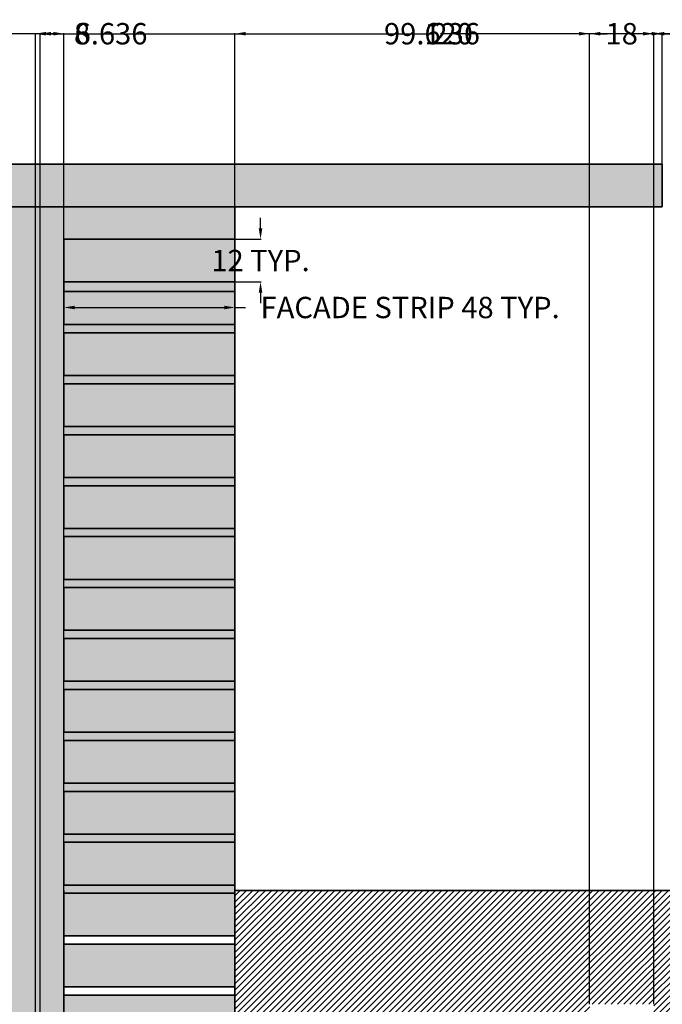
# Model space of a CAD drawing. Units: inches. Extents: x 126 to 726, y 86 to 888.
# Tile 12 of 13: x 426 to 606, y 611 to 888. Entities that reach past the tile are written whole.
import ezdxf

# ---------------------------------------------------------------- set-up
doc = ezdxf.new("R2010")
doc.units = ezdxf.units.IN
doc.header["$MEASUREMENT"] = 0
for name, color, linetype, lineweight in [('A-ANNO-DIMS', 2, 'Continuous', 18), ('A-ELEV', 7, 'Continuous', 35), ('A-ELEV-PATT', 8, 'Continuous', 13)]:
    doc.layers.add(name, color=color, linetype=linetype, lineweight=lineweight)
doc.styles.get("Standard").update_dxf_attribs({"font": 'arial.ttf'})
doc.dimstyles.get("Standard").update_dxf_attribs({"dimtxt": 6, "dimasz": 3, "dimexe": 0.18, "dimexo": 0.0625, "dimgap": 0.09, "dimtad": 0, "dimtih": 1, "dimtoh": 1, "dimdec": 0, "dimzin": 0, "dimdsep": 46, "dimlunit": 3, "dimtxsty": 'Standard', "dimcen": 0.09, "dimadec": 0, "dimazin": 0, "dimtfac": 1, "dimtdec": 0, "dimtofl": 0, "dimtmove": 0, "dimatfit": 3, "dimfxl": 1, "dimtolj": 1, "dimtzin": 0, "dimarcsym": 0})

# ---------------------------------------------------------------- blocks, each defined once
blk = doc.blocks.new('FACADE-STRIP')
for p, q in [((0, 0), (0, 12)), ((0, 12), (48, 12)), ((0, 0), (48, 0))]:
    blk.add_line(p, q)
blk = doc.blocks.new('*D11')
at = {"layer": 'A-ANNO-DIMS', "color": 0, "lineweight": -2, "transparency": 16777216}
for p, q in [((437.97, 813.91), (437.97, 806.6)), ((485.97, 813.91), (485.97, 806.6)), ((440.97, 806.78), (482.97, 806.78)), ((485.97, 806.78), (488.97, 806.78))]:
    blk.add_line(p, q, dxfattribs=at)
at = {"layer": 'A-ANNO-DIMS', "color": 0, "transparency": 16777216}
for points in [[(440.97, 807.28), (440.97, 806.28), (437.97, 806.78)], [(482.97, 807.28), (482.97, 806.28), (485.97, 806.78)]]:
    blk.add_solid(points, dxfattribs=at)
at = {"layer": 'Defpoints', "color": 0, "transparency": 16777216}
for p in [(437.97, 813.98), (485.97, 813.98), (485.97, 806.78)]:
    blk.add_point(p, dxfattribs=at)
at = {"layer": 'A-ANNO-DIMS', "color": 0, "transparency": 16777216, "insert": (535.17, 806.78), "char_height": 6, "attachment_point": 5}
blk.add_mtext('\\A1;FACADE STRIP 48 TYP.', dxfattribs=at)
blk = doc.blocks.new('*D12')
at = {"layer": 'A-ANNO-DIMS', "color": 0, "lineweight": -2, "transparency": 16777216}
for p, q in [((493.17, 828.98), (493.17, 831.98)), ((486.04, 825.98), (493.35, 825.98)), ((486.04, 813.98), (493.35, 813.98)), ((493.17, 810.98), (493.17, 807.98))]:
    blk.add_line(p, q, dxfattribs=at)
at = {"layer": 'A-ANNO-DIMS', "color": 0, "transparency": 16777216}
for points in [[(492.67, 828.98), (493.67, 828.98), (493.17, 825.98)], [(492.67, 810.98), (493.67, 810.98), (493.17, 813.98)]]:
    blk.add_solid(points, dxfattribs=at)
at = {"layer": 'Defpoints', "color": 0, "transparency": 16777216}
for p in [(485.97, 825.98), (493.17, 825.98), (485.97, 813.98)]:
    blk.add_point(p, dxfattribs=at)
at = {"layer": 'A-ANNO-DIMS', "color": 0, "transparency": 16777216, "insert": (493.17, 819.98), "char_height": 6, "attachment_point": 5}
blk.add_mtext('\\A1;12 TYP.', dxfattribs=at)
blk = doc.blocks.new('*D13')
at = {"layer": 'A-ANNO-DIMS', "color": 0, "lineweight": -2, "transparency": 16777216}
for p, q in [((665.97, 642.98), (665.97, 90.21)), ((185.97, 126.98), (185.97, 90.21)), ((188.97, 90.39), (419.15, 90.39)), ((662.97, 90.39), (432.8, 90.39))]:
    blk.add_line(p, q, dxfattribs=at)
at = {"layer": 'A-ANNO-DIMS', "color": 0, "transparency": 16777216}
for points in [[(188.97, 90.89), (188.97, 89.89), (185.97, 90.39)], [(662.97, 90.89), (662.97, 89.89), (665.97, 90.39)]]:
    blk.add_solid(points, dxfattribs=at)
at = {"layer": 'Defpoints', "color": 0, "transparency": 16777216}
for p in [(665.97, 643.04), (185.97, 127.04), (665.97, 90.39)]:
    blk.add_point(p, dxfattribs=at)
at = {"layer": 'A-ANNO-DIMS', "color": 0, "transparency": 16777216, "insert": (425.97, 90.39), "char_height": 6, "attachment_point": 5}
blk.add_mtext('\\A1;480', dxfattribs=at)
blk = doc.blocks.new('*D22')
at = {"layer": 'A-ANNO-DIMS', "color": 0, "lineweight": -2, "transparency": 16777216}
for p, q in [((185.91, 847.04), (149.14, 847.04)), ((149.32, 844.04), (149.32, 708.47)), ((149.32, 566.58), (149.32, 702.16)), ((431.28, 563.58), (149.14, 563.58))]:
    blk.add_line(p, q, dxfattribs=at)
at = {"layer": 'A-ANNO-DIMS', "color": 0, "transparency": 16777216}
for points in [[(148.82, 844.04), (149.82, 844.04), (149.32, 847.04)], [(148.82, 566.58), (149.82, 566.58), (149.32, 563.58)]]:
    blk.add_solid(points, dxfattribs=at)
at = {"layer": 'Defpoints', "color": 0, "transparency": 16777216}
for p in [(149.32, 847.04), (185.97, 847.04), (431.34, 563.58)]:
    blk.add_point(p, dxfattribs=at)
at = {"layer": 'A-ANNO-DIMS', "color": 0, "transparency": 16777216, "insert": (149.32, 705.31), "char_height": 6, "attachment_point": 5}
blk.add_mtext('\\A1;283.46', dxfattribs=at)
blk = doc.blocks.new('*D25')
at = {"layer": 'A-ANNO-DIMS', "color": 0, "lineweight": -2, "transparency": 16777216}
for p, q in [((371.32, 763.42), (371.32, 883.87)), ((374.32, 883.69), (394.42, 883.69)), ((434.97, 883.69), (414.87, 883.69)), ((437.97, 826.04), (437.97, 883.87))]:
    blk.add_line(p, q, dxfattribs=at)
at = {"layer": 'A-ANNO-DIMS', "color": 0, "transparency": 16777216}
for points in [[(374.32, 884.19), (374.32, 883.19), (371.32, 883.69)], [(434.97, 884.19), (434.97, 883.19), (437.97, 883.69)]]:
    blk.add_solid(points, dxfattribs=at)
at = {"layer": 'Defpoints', "color": 0, "transparency": 16777216}
for p in [(437.97, 883.69), (437.97, 825.98), (371.32, 763.35)]:
    blk.add_point(p, dxfattribs=at)
at = {"layer": 'A-ANNO-DIMS', "color": 0, "transparency": 16777216, "insert": (404.65, 883.69), "char_height": 6, "attachment_point": 5}
blk.add_mtext('\\A1;66.66', dxfattribs=at)
blk = doc.blocks.new('*D26')
at = {"layer": 'A-ANNO-DIMS', "color": 0, "lineweight": -2, "transparency": 16777216}
for p, q in [((485.97, 835.1), (485.97, 883.87)), ((488.97, 883.69), (539.55, 883.69)), ((602.97, 883.69), (552.4, 883.69)), ((605.97, 835.1), (605.97, 883.87))]:
    blk.add_line(p, q, dxfattribs=at)
at = {"layer": 'A-ANNO-DIMS', "color": 0, "transparency": 16777216}
for points in [[(488.97, 884.19), (488.97, 883.19), (485.97, 883.69)], [(602.97, 884.19), (602.97, 883.19), (605.97, 883.69)]]:
    blk.add_solid(points, dxfattribs=at)
at = {"layer": 'Defpoints', "color": 0, "transparency": 16777216}
for p in [(605.97, 883.69), (485.97, 835.04), (605.97, 835.04)]:
    blk.add_point(p, dxfattribs=at)
at = {"layer": 'A-ANNO-DIMS', "color": 0, "transparency": 16777216, "insert": (545.97, 883.69), "char_height": 6, "attachment_point": 5}
blk.add_mtext('\\A1;120', dxfattribs=at)
blk = doc.blocks.new('*D41')
at = {"layer": 'A-ANNO-DIMS', "color": 0, "lineweight": -2, "transparency": 16777216}
for p, q in [((429.97, 607.1), (429.97, 883.87)), ((432.97, 883.69), (541.21, 883.69)), ((662.97, 883.69), (554.74, 883.69)), ((665.97, 607.1), (665.97, 883.87))]:
    blk.add_line(p, q, dxfattribs=at)
at = {"layer": 'A-ANNO-DIMS', "color": 0, "transparency": 16777216}
for points in [[(432.97, 884.19), (432.97, 883.19), (429.97, 883.69)], [(662.97, 884.19), (662.97, 883.19), (665.97, 883.69)]]:
    blk.add_solid(points, dxfattribs=at)
at = {"layer": 'Defpoints', "color": 0, "transparency": 16777216}
for p in [(665.97, 883.69), (429.97, 607.04), (665.97, 607.04)]:
    blk.add_point(p, dxfattribs=at)
at = {"layer": 'A-ANNO-DIMS', "color": 0, "transparency": 16777216, "insert": (547.97, 883.69), "char_height": 6, "attachment_point": 5}
blk.add_mtext('\\A1;236', dxfattribs=at)
blk = doc.blocks.new('*D43')
at = {"layer": 'A-ANNO-DIMS', "color": 0, "lineweight": -2, "transparency": 16777216}
for p, q in [((429.97, 595.1), (429.97, 883.87)), ((432.97, 883.69), (434.97, 883.69)), ((437.97, 585.06), (437.97, 883.87)), ((437.97, 883.69), (440.97, 883.69))]:
    blk.add_line(p, q, dxfattribs=at)
at = {"layer": 'A-ANNO-DIMS', "color": 0, "transparency": 16777216}
for points in [[(432.97, 884.19), (432.97, 883.19), (429.97, 883.69)], [(434.97, 884.19), (434.97, 883.19), (437.97, 883.69)]]:
    blk.add_solid(points, dxfattribs=at)
at = {"layer": 'Defpoints', "color": 0, "transparency": 16777216}
for p in [(437.97, 883.69), (429.97, 595.04), (437.97, 585)]:
    blk.add_point(p, dxfattribs=at)
at = {"layer": 'A-ANNO-DIMS', "color": 0, "transparency": 16777216, "insert": (443.04, 883.69), "char_height": 6, "attachment_point": 5}
blk.add_mtext('\\A1;8', dxfattribs=at)
blk = doc.blocks.new('*D44')
at = {"layer": 'A-ANNO-DIMS', "color": 0, "lineweight": -2, "transparency": 16777216}
for p, q in [((431.34, 563.65), (431.34, 883.87)), ((434.34, 883.69), (434.97, 883.69)), ((437.97, 570.75), (437.97, 883.87)), ((437.97, 883.69), (440.97, 883.69))]:
    blk.add_line(p, q, dxfattribs=at)
at = {"layer": 'A-ANNO-DIMS', "color": 0, "transparency": 16777216}
for points in [[(434.34, 884.19), (434.34, 883.19), (431.34, 883.69)], [(434.97, 884.19), (434.97, 883.19), (437.97, 883.69)]]:
    blk.add_solid(points, dxfattribs=at)
at = {"layer": 'Defpoints', "color": 0, "transparency": 16777216}
for p in [(437.97, 883.69), (437.97, 570.69), (431.34, 563.58)]:
    blk.add_point(p, dxfattribs=at)
at = {"layer": 'A-ANNO-DIMS', "color": 0, "transparency": 16777216, "insert": (451.2, 883.69), "char_height": 6, "attachment_point": 5}
blk.add_mtext('\\A1;6.636', dxfattribs=at)
blk = doc.blocks.new('*D50')
at = {"layer": 'A-ANNO-DIMS', "color": 0, "lineweight": -2, "transparency": 16777216}
for p, q in [((485.97, 643.1), (485.97, 883.87)), ((488.97, 883.69), (527.9, 883.69)), ((582.58, 883.69), (543.66, 883.69)), ((585.58, 611.1), (585.58, 883.87))]:
    blk.add_line(p, q, dxfattribs=at)
at = {"layer": 'A-ANNO-DIMS', "color": 0, "transparency": 16777216}
for points in [[(488.97, 884.19), (488.97, 883.19), (485.97, 883.69)], [(582.58, 884.19), (582.58, 883.19), (585.58, 883.69)]]:
    blk.add_solid(points, dxfattribs=at)
at = {"layer": 'Defpoints', "color": 0, "transparency": 16777216}
for p in [(585.58, 883.69), (485.97, 643.04), (585.58, 611.04)]:
    blk.add_point(p, dxfattribs=at)
at = {"layer": 'A-ANNO-DIMS', "color": 0, "transparency": 16777216, "insert": (535.78, 883.69), "char_height": 6, "attachment_point": 5}
blk.add_mtext('\\A1;99.6', dxfattribs=at)
blk = doc.blocks.new('*D51')
at = {"layer": 'A-ANNO-DIMS', "color": 0, "lineweight": -2, "transparency": 16777216}
for p, q in [((585.58, 611.1), (585.58, 883.87)), ((588.58, 883.69), (590.47, 883.69)), ((600.58, 883.69), (598.69, 883.69)), ((603.58, 611.1), (603.58, 883.87))]:
    blk.add_line(p, q, dxfattribs=at)
at = {"layer": 'A-ANNO-DIMS', "color": 0, "transparency": 16777216}
for points in [[(588.58, 884.19), (588.58, 883.19), (585.58, 883.69)], [(600.58, 884.19), (600.58, 883.19), (603.58, 883.69)]]:
    blk.add_solid(points, dxfattribs=at)
at = {"layer": 'Defpoints', "color": 0, "transparency": 16777216}
for p in [(603.58, 883.69), (585.58, 611.04), (603.58, 611.04)]:
    blk.add_point(p, dxfattribs=at)
at = {"layer": 'A-ANNO-DIMS', "color": 0, "transparency": 16777216, "insert": (594.58, 883.69), "char_height": 6, "attachment_point": 5}
blk.add_mtext('\\A1;18', dxfattribs=at)
blk = doc.blocks.new('*D52')
at = {"layer": 'A-ANNO-DIMS', "color": 0, "lineweight": -2, "transparency": 16777216}
for p, q in [((603.58, 611.1), (603.58, 883.87)), ((606.58, 883.69), (608.58, 883.69)), ((611.58, 611.1), (611.58, 883.87)), ((611.58, 883.69), (614.58, 883.69))]:
    blk.add_line(p, q, dxfattribs=at)
at = {"layer": 'A-ANNO-DIMS', "color": 0, "transparency": 16777216}
for points in [[(606.58, 884.19), (606.58, 883.19), (603.58, 883.69)], [(608.58, 884.19), (608.58, 883.19), (611.58, 883.69)]]:
    blk.add_solid(points, dxfattribs=at)
at = {"layer": 'Defpoints', "color": 0, "transparency": 16777216}
for p in [(611.58, 883.69), (603.58, 611.04), (611.58, 611.04)]:
    blk.add_point(p, dxfattribs=at)
at = {"layer": 'A-ANNO-DIMS', "color": 0, "transparency": 16777216, "insert": (616.65, 883.69), "char_height": 6, "attachment_point": 5}
blk.add_mtext('\\A1;8', dxfattribs=at)

msp = doc.modelspace()

# ---------------------------------------------------------------- hatches: boundary and pattern name
at = {"layer": 'A-ELEV-PATT'}
h = msp.add_hatch(color=256, dxfattribs=at)
h.dxf.hatch_style = 1
h.paths.add_polyline_path([(233.9749, 545.5846), (431.3386, 545.5846), (431.3386, 563.5846), (185.9749, 563.5846), (185.9749, 395.5846), (431.3386, 395.5846), (431.3386, 413.5846), (233.9749, 413.5846)])
h.paths.add_polyline_path([(233.9749, 835.0424), (485.9749, 835.0424), (605.9749, 835.0424), (605.9749, 847.0424), (485.9749, 847.0424), (185.9749, 847.0424), (185.9749, 606.5846), (233.9749, 606.5846)])
h.paths.add_polyline_path([(233.9749, 597.5846), (185.9749, 597.5846), (185.9749, 585.5846), (233.9749, 585.5846)])
h.paths.add_polyline_path([(233.9749, 580.5846), (185.9749, 580.5846), (185.9749, 568.5846), (233.9749, 568.5846)])
h = msp.add_hatch(color=256, dxfattribs=at)
h.dxf.hatch_style = 1
h.paths.add_polyline_path([(437.9749, 499.1312), (485.9749, 499.1312), (485.9749, 501.4423), (437.9749, 501.4423), (437.9749, 513.4423), (485.9749, 513.4423), (485.9749, 515.7534), (437.9749, 515.7534), (437.9749, 527.7534), (485.9749, 527.7534), (485.9749, 530.0646), (437.9749, 530.0646), (437.9749, 542.0646), (485.9749, 542.0646), (485.9749, 544.3757), (437.9749, 544.3757), (437.9749, 556.3757), (485.9749, 556.3757), (485.9749, 558.6868), (437.9749, 558.6868), (437.9749, 570.6868), (485.9749, 570.6868), (485.9749, 572.9979), (437.9749, 572.9979), (437.9749, 584.9979), (485.9749, 584.9979), (485.9749, 587.309), (437.9749, 587.309), (437.9749, 595.0424), (429.9749, 595.0424), (429.9749, 607.0424), (437.9749, 607.0424), (437.9749, 615.9312), (437.9749, 630.2423), (437.9749, 642.2423), (485.9749, 642.2423), (485.9749, 644.5534), (437.9749, 644.5534), (437.9749, 656.5534), (485.9749, 656.5534), (485.9749, 658.8645), (437.9749, 658.8645), (437.9749, 670.8645), (485.9749, 670.8645), (485.9749, 673.1757), (437.9749, 673.1757), (437.9749, 685.1757), (485.9749, 685.1757), (485.9749, 687.4868), (437.9749, 687.4868), (437.9749, 699.4868), (485.9749, 699.4868), (485.9749, 701.7979), (437.9749, 701.7979), (437.9749, 713.7979), (485.9749, 713.7979), (485.9749, 716.109), (437.9749, 716.109), (437.9749, 728.109), (485.9749, 728.109), (485.9749, 730.4201), (437.9749, 730.4201), (437.9749, 742.4201), (485.9749, 742.4201), (485.9749, 744.7312), (437.9749, 744.7312), (437.9749, 756.7312), (485.9749, 756.7312), (485.9749, 759.0423), (437.9749, 759.0423), (437.9749, 771.0423), (485.9749, 771.0423), (485.9749, 773.3534), (437.9749, 773.3534), (437.9749, 785.3534), (485.9749, 785.3534), (485.9749, 787.6645), (437.9749, 787.6645), (437.9749, 799.6645), (485.9749, 799.6645), (485.9749, 801.9756), (437.9749, 801.9756), (437.9749, 811.2868), (485.9749, 811.2868), (485.9749, 813.9756), (437.9749, 813.9756), (437.9749, 825.9756), (485.9749, 825.9756), (485.9749, 835.0424), (233.9749, 835.0424), (233.9749, 606.5846), (185.9749, 606.5846), (185.9749, 597.5846), (233.9749, 597.5846), (233.9749, 585.5846), (185.9749, 585.5846), (185.9749, 580.5846), (233.9749, 580.5846), (233.9749, 568.5846), (185.9749, 568.5846), (185.9749, 563.5846), (431.3386, 563.5846), (431.3386, 545.5846), (233.9749, 545.5846), (233.9749, 413.5846), (431.3386, 413.5846), (431.3386, 395.5846), (185.9749, 395.5846), (185.9749, 386.5846), (233.9749, 386.5846), (233.9749, 374.5846), (185.9749, 374.5846), (185.9749, 369.5846), (233.9749, 369.5846), (233.9749, 357.5846), (185.9749, 357.5846), (185.9749, 352.5846), (233.9749, 352.5846), (233.9749, 340.5846), (185.9749, 340.5846), (185.9749, 331.5846), (233.9749, 331.5846), (233.9749, 127.0424), (485.9749, 127.0424), (485.9749, 129.3535), (437.9749, 129.3535), (437.9749, 141.3535), (485.9749, 141.3535), (485.9749, 143.6646), (437.9749, 143.6646), (437.9749, 155.6646), (485.9749, 155.6646), (485.9749, 157.9757), (437.9749, 157.9757), (437.9749, 169.9757), (485.9749, 169.9757), (485.9749, 172.2868), (437.9749, 172.2868), (437.9749, 184.2868), (485.9749, 184.2868), (485.9749, 186.5979), (437.9749, 186.5979), (437.9749, 198.5979), (485.9749, 198.5979), (485.9749, 200.909), (437.9749, 200.909), (437.9749, 212.909), (485.9749, 212.909), (485.9749, 215.2201), (437.9749, 215.2201), (437.9749, 227.2201), (485.9749, 227.2201), (485.9749, 229.5312), (437.9749, 229.5312), (437.9749, 241.5312), (485.9749, 241.5312), (485.9749, 243.8424), (437.9749, 243.8424), (437.9749, 255.8424), (485.9749, 255.8424), (485.9749, 258.1535), (437.9749, 258.1535), (437.9749, 270.1535), (485.9749, 270.1535), (485.9749, 272.4646), (437.9749, 272.4646), (437.9749, 284.4646), (485.9749, 284.4646), (485.9749, 286.7757), (437.9749, 286.7757), (437.9749, 298.7757), (485.9749, 298.7757), (485.9749, 301.0868), (437.9749, 301.0868), (437.9749, 313.0868), (485.9749, 313.0868), (485.9749, 315.3979), (437.9749, 315.3979), (437.9749, 327.3979), (485.9749, 327.3979), (485.9749, 329.709), (437.9749, 329.709), (437.9749, 341.709), (485.9749, 341.709), (485.9749, 344.0201), (437.9749, 344.0201), (437.9749, 355.0424), (429.9749, 355.0424), (429.9749, 367.0424), (437.9749, 367.0424), (437.9749, 372.6423), (437.9749, 386.9535), (437.9749, 401.2646), (437.9749, 413.2646), (485.9749, 413.2646), (485.9749, 415.5757), (437.9749, 415.5757), (437.9749, 427.5757), (485.9749, 427.5757), (485.9749, 429.8868), (437.9749, 429.8868), (437.9749, 441.8868), (485.9749, 441.8868), (485.9749, 444.1979), (437.9749, 444.1979), (437.9749, 456.1979), (485.9749, 456.1979), (485.9749, 458.509), (437.9749, 458.509), (437.9749, 470.509), (485.9749, 470.509), (485.9749, 472.8201), (437.9749, 472.8201), (437.9749, 484.8201), (485.9749, 484.8201), (485.9749, 487.1312), (437.9749, 487.1312)])
h.paths.add_polyline_path([(299.6658, 533.6845), (371.6658, 533.6845), (371.6658, 425.6845), (299.6658, 425.6845)], flags=16)
h.paths.add_polyline_path([(308.6658, 524.6845), (362.6658, 524.6845), (362.6658, 434.6845), (308.6658, 434.6845)], flags=0)
h.paths.add_polyline_path([(317.7956, 603.3211, -0.4129833), (306.8418, 614.321, -0.94403766), (328.769, 615.5845, -0.04423165), (330.7031, 615.4048, -0.89973713), (352.5798, 615.6161, -0.4129833), (363.5336, 604.6162, -0.94403766), (341.6064, 603.3528, -0.04423165), (339.6723, 603.5324, -0.89973713)], flags=16)
h.paths.add_polyline_path([(319.7228, 604.5846, -0.02633223), (319.7726, 605.5306, -0.47905713), (308.8418, 614.321, -1), (326.8418, 614.321, -0.02633223), (326.7919, 613.375, -0.17413188), (332.826, 612.5948, -0.04918553), (332.6526, 614.3527, -1), (350.6526, 614.3527, -0.02633223), (350.6028, 613.4067, -0.47905713), (361.5336, 604.6162, -1), (343.5336, 604.6162, -0.02633223), (343.5834, 605.5622, -0.17413188), (337.5494, 606.3424, -0.04918553), (337.7228, 604.5846, -1)], flags=0)
h.paths.add_polyline_path([(328.769, 355.6561, -0.04423165), (330.7031, 355.4765, -0.89973713), (352.5798, 355.6878, -0.4129833), (363.5336, 344.6879, -0.94403766), (341.6064, 343.4244, -0.04423165), (339.6723, 343.604, -0.89973713), (317.7956, 343.3927, -0.4129833), (306.8418, 354.3926, -0.94403766)], flags=16)
h.paths.add_polyline_path([(326.8418, 354.3926, -0.02633223), (326.7919, 353.4466, -0.17413188), (332.826, 352.6664, -0.04918553), (332.6526, 354.4243, -1), (350.6526, 354.4243, -0.02633223), (350.6028, 353.4783, -0.47905713), (361.5336, 344.6879, -1), (343.5336, 344.6879, -0.02633223), (343.5834, 345.6339, -0.17413188), (337.5494, 346.4141, -0.04918553), (337.7228, 344.6562, -1), (319.7228, 344.6562, -0.02633223), (319.7726, 345.6022, -0.47905713), (308.8418, 354.3926, -1)], flags=0)
h.paths.add_polyline_path([(299.3189, 655.3527), (299.3189, 763.3527), (371.3189, 763.3527), (371.3189, 655.3527)], flags=16)
h.paths.add_polyline_path([(308.3189, 664.3527), (308.3189, 754.3527), (362.3189, 754.3527), (362.3189, 664.3527)], flags=0)
h.paths.add_polyline_path([(299.6658, 303.5875), (371.6658, 303.5875), (371.6658, 195.5875), (299.6658, 195.5875)], flags=16)
h.paths.add_polyline_path([(308.6658, 294.5875), (362.6658, 294.5875), (362.6658, 204.5875), (308.6658, 204.5875)], flags=0)
h.paths.add_polyline_path([(326.3038, 177.3867), (346.055, 177.3867, -0.41421356), (349.055, 174.3867), (349.055, 171.2378), (363.489, 171.2378, -0.41421356), (366.489, 168.2378), (366.489, 159.7133, -0.41421356), (363.489, 156.7133), (343.7379, 156.7133, -0.41421356), (340.7379, 159.7133), (340.7379, 162.8622), (330.5504, 162.8622), (330.5504, 159.7133, -0.41421356), (327.5504, 156.7133), (307.7992, 156.7133, -0.41421356), (304.7992, 159.7133), (304.7992, 168.2378, -0.41421356), (307.7992, 171.2378), (323.3038, 171.2378), (323.3038, 174.3867, -0.41421356)], flags=16)
h.paths.add_polyline_path([(326.3038, 175.3867), (346.055, 175.3867, -0.41421356), (347.055, 174.3867), (347.055, 169.2378), (363.489, 169.2378, -0.41421356), (364.489, 168.2378), (364.489, 159.7133, -0.41421356), (363.489, 158.7133), (343.7379, 158.7133, -0.41421356), (342.7379, 159.7133), (342.7379, 164.8622), (328.5504, 164.8622), (328.5504, 159.7133, -0.41421356), (327.5504, 158.7133), (307.7992, 158.7133, -0.41421356), (306.7992, 159.7133), (306.7992, 168.2378, -0.41421356), (307.7992, 169.2378), (325.3038, 169.2378), (325.3038, 174.3867, -0.41421356)], flags=0)
h = msp.add_hatch(dxfattribs=at)
h.set_pattern_fill('GRAVEL', color=256, scale=40)
h.paths.add_polyline_path([(437.9749, 642.2423), (485.9749, 642.2423), (485.9749, 644.5534), (437.9749, 644.5534), (437.9749, 656.5534), (485.9749, 656.5534), (485.9749, 658.8645), (437.9749, 658.8645), (437.9749, 670.8645), (485.9749, 670.8645), (485.9749, 673.1757), (437.9749, 673.1757), (437.9749, 685.1757), (485.9749, 685.1757), (485.9749, 687.4868), (437.9749, 687.4868), (437.9749, 699.4868), (485.9749, 699.4868), (485.9749, 701.7979), (437.9749, 701.7979), (437.9749, 713.7979), (485.9749, 713.7979), (485.9749, 716.109), (437.9749, 716.109), (437.9749, 728.109), (485.9749, 728.109), (485.9749, 730.4201), (437.9749, 730.4201), (437.9749, 742.4201), (485.9749, 742.4201), (485.9749, 744.7312), (437.9749, 744.7312), (437.9749, 756.7312), (485.9749, 756.7312), (485.9749, 759.0423), (437.9749, 759.0423), (437.9749, 771.0423), (485.9749, 771.0423), (485.9749, 773.3534), (437.9749, 773.3534), (437.9749, 785.3534), (485.9749, 785.3534), (485.9749, 787.6645), (437.9749, 787.6645), (437.9749, 799.6645), (485.9749, 799.6645), (485.9749, 801.9756), (437.9749, 801.9756), (437.9749, 811.2868), (485.9749, 811.2868), (485.9749, 813.9756), (437.9749, 813.9756), (437.9749, 825.9756), (485.9749, 825.9756), (485.9749, 835.0424), (233.9749, 835.0424), (233.9749, 606.5846), (185.9749, 606.5846), (185.9749, 597.5846), (233.9749, 597.5846), (233.9749, 585.5846), (185.9749, 585.5846), (185.9749, 580.5846), (233.9749, 580.5846), (233.9749, 568.5846), (185.9749, 568.5846), (185.9749, 563.5846), (431.3386, 563.5846), (431.3386, 545.5846), (233.9749, 545.5846), (233.9749, 413.5846), (431.3386, 413.5846), (431.3386, 395.5846), (185.9749, 395.5846), (185.9749, 386.5846), (233.9749, 386.5846), (233.9749, 374.5846), (185.9749, 374.5846), (185.9749, 369.5846), (233.9749, 369.5846), (233.9749, 357.5846), (185.9749, 357.5846), (185.9749, 352.5846), (233.9749, 352.5846), (233.9749, 340.5846), (185.9749, 340.5846), (185.9749, 331.5846), (233.9749, 331.5846), (233.9749, 127.0424), (485.9749, 127.0424), (485.9749, 129.3535), (437.9749, 129.3535), (437.9749, 141.3535), (485.9749, 141.3535), (485.9749, 143.6646), (437.9749, 143.6646), (437.9749, 155.6646), (485.9749, 155.6646), (485.9749, 157.9757), (437.9749, 157.9757), (437.9749, 169.9757), (485.9749, 169.9757), (485.9749, 172.2868), (437.9749, 172.2868), (437.9749, 184.2868), (485.9749, 184.2868), (485.9749, 186.5979), (437.9749, 186.5979), (437.9749, 198.5979), (485.9749, 198.5979), (485.9749, 200.909), (437.9749, 200.909), (437.9749, 212.909), (485.9749, 212.909), (485.9749, 215.2201), (437.9749, 215.2201), (437.9749, 227.2201), (485.9749, 227.2201), (485.9749, 229.5312), (437.9749, 229.5312), (437.9749, 241.5312), (485.9749, 241.5312), (485.9749, 243.8424), (437.9749, 243.8424), (437.9749, 255.8424), (485.9749, 255.8424), (485.9749, 258.1535), (437.9749, 258.1535), (437.9749, 270.1535), (485.9749, 270.1535), (485.9749, 272.4646), (437.9749, 272.4646), (437.9749, 284.4646), (485.9749, 284.4646), (485.9749, 286.7757), (437.9749, 286.7757), (437.9749, 298.7757), (485.9749, 298.7757), (485.9749, 301.0868), (437.9749, 301.0868), (437.9749, 313.0868), (485.9749, 313.0868), (485.9749, 315.3979), (437.9749, 315.3979), (437.9749, 327.3979), (485.9749, 327.3979), (485.9749, 329.709), (437.9749, 329.709), (437.9749, 341.709), (485.9749, 341.709), (485.9749, 344.0201), (437.9749, 344.0201), (437.9749, 355.0424), (429.9749, 355.0424), (429.9749, 367.0424), (437.9749, 367.0424), (437.9749, 372.6423), (437.9749, 386.9535), (437.9749, 401.2646), (437.9749, 413.2646), (485.9749, 413.2646), (485.9749, 415.5757), (437.9749, 415.5757), (437.9749, 427.5757), (485.9749, 427.5757), (485.9749, 429.8868), (437.9749, 429.8868), (437.9749, 441.8868), (485.9749, 441.8868), (485.9749, 444.1979), (437.9749, 444.1979), (437.9749, 456.1979), (485.9749, 456.1979), (485.9749, 458.509), (437.9749, 458.509), (437.9749, 470.509), (485.9749, 470.509), (485.9749, 472.8201), (437.9749, 472.8201), (437.9749, 484.8201), (485.9749, 484.8201), (485.9749, 487.1312), (437.9749, 487.1312), (437.9749, 499.1312), (485.9749, 499.1312), (485.9749, 501.4423), (437.9749, 501.4423), (437.9749, 513.4423), (485.9749, 513.4423), (485.9749, 515.7534), (437.9749, 515.7534), (437.9749, 527.7534), (485.9749, 527.7534), (485.9749, 530.0646), (437.9749, 530.0646), (437.9749, 542.0646), (485.9749, 542.0646), (485.9749, 544.3757), (437.9749, 544.3757), (437.9749, 556.3757), (485.9749, 556.3757), (485.9749, 558.6868), (437.9749, 558.6868), (437.9749, 570.6868), (485.9749, 570.6868), (485.9749, 572.9979), (437.9749, 572.9979), (437.9749, 584.9979), (485.9749, 584.9979), (485.9749, 587.309), (437.9749, 587.309), (437.9749, 595.0424), (429.9749, 595.0424), (429.9749, 607.0424), (437.9749, 607.0424), (437.9749, 615.9312), (437.9749, 630.2423)])
h.paths.add_polyline_path([(371.3189, 655.3527), (299.3189, 655.3527), (299.3189, 763.3527), (371.3189, 763.3527)], flags=16)
h.paths.add_polyline_path([(363.5336, 604.6162, -0.94403766), (341.6064, 603.3528, -0.04423165), (339.6723, 603.5324, -0.89973713), (317.7956, 603.3211, -0.4129833), (306.8418, 614.321, -0.94403766), (328.769, 615.5845, -0.04423165), (330.7031, 615.4048, -0.89973713), (352.5798, 615.6161, -0.4129833)], flags=16)
h.paths.add_polyline_path([(361.5336, 604.6162, -1), (343.5336, 604.6162, -0.02633223), (343.5834, 605.5622, -0.17413188), (337.5494, 606.3424, -0.04918553), (337.7228, 604.5846, -1), (319.7228, 604.5846, -0.02633223), (319.7726, 605.5306, -0.47905713), (308.8418, 614.321, -1), (326.8418, 614.321, -0.02633223), (326.7919, 613.375, -0.17413188), (332.826, 612.5948, -0.04918553), (332.6526, 614.3527, -1), (350.6526, 614.3527, -0.02633223), (350.6028, 613.4067, -0.47905713)], flags=0)
h.paths.add_polyline_path([(362.3189, 664.3527), (308.3189, 664.3527), (308.3189, 754.3527), (362.3189, 754.3527)], flags=0)
h.paths.add_polyline_path([(371.6658, 533.6845), (371.6658, 425.6845), (299.6658, 425.6845), (299.6658, 533.6845)], flags=16)
h.paths.add_polyline_path([(362.6658, 524.6845), (362.6658, 434.6845), (308.6658, 434.6845), (308.6658, 524.6845)], flags=0)
h.paths.add_polyline_path([(352.5798, 355.6878, -0.4129833), (363.5336, 344.6879, -0.94403766), (341.6064, 343.4244, -0.04423165), (339.6723, 343.604, -0.89973713), (317.7956, 343.3927, -0.4129833), (306.8418, 354.3926, -0.94403766), (328.769, 355.6561, -0.04423165), (330.7031, 355.4765, -0.89973713)], flags=16)
h.paths.add_polyline_path([(350.6526, 354.4243, -0.02633223), (350.6028, 353.4783, -0.47905713), (361.5336, 344.6879, -1), (343.5336, 344.6879, -0.02633223), (343.5834, 345.6339, -0.17413188), (337.5494, 346.4141, -0.04918553), (337.7228, 344.6562, -1), (319.7228, 344.6562, -0.02633223), (319.7726, 345.6022, -0.47905713), (308.8418, 354.3926, -1), (326.8418, 354.3926, -0.02633223), (326.7919, 353.4466, -0.17413188), (332.826, 352.6664, -0.04918553), (332.6526, 354.4243, -1)], flags=0)
h.paths.add_polyline_path([(371.6658, 303.5875), (371.6658, 195.5875), (299.6658, 195.5875), (299.6658, 303.5875)], flags=16)
h.paths.add_polyline_path([(362.6658, 294.5875), (362.6658, 204.5875), (308.6658, 204.5875), (308.6658, 294.5875)], flags=0)
h.paths.add_polyline_path([(346.055, 177.3867, -0.41421356), (349.055, 174.3867), (349.055, 171.2378), (363.489, 171.2378, -0.41421356), (366.489, 168.2378), (366.489, 159.7133, -0.41421356), (363.489, 156.7133), (343.7379, 156.7133, -0.41421356), (340.7379, 159.7133), (340.7379, 162.8622), (330.5504, 162.8622), (330.5504, 159.7133, -0.41421356), (327.5504, 156.7133), (307.7992, 156.7133, -0.41421356), (304.7992, 159.7133), (304.7992, 168.2378, -0.41421356), (307.7992, 171.2378), (323.3038, 171.2378), (323.3038, 174.3867, -0.41421356), (326.3038, 177.3867)], flags=16)
h.paths.add_polyline_path([(346.055, 175.3867, -0.41421356), (347.055, 174.3867), (347.055, 169.2378), (363.489, 169.2378, -0.41421356), (364.489, 168.2378), (364.489, 159.7133, -0.41421356), (363.489, 158.7133), (343.7379, 158.7133, -0.41421356), (342.7379, 159.7133), (342.7379, 164.8622), (328.5504, 164.8622), (328.5504, 159.7133, -0.41421356), (327.5504, 158.7133), (307.7992, 158.7133, -0.41421356), (306.7992, 159.7133), (306.7992, 168.2378, -0.41421356), (307.7992, 169.2378), (325.3038, 169.2378), (325.3038, 174.3867, -0.41421356), (326.3038, 175.3867)], flags=0)
h = msp.add_hatch(color=256, dxfattribs=at)
h.dxf.hatch_style = 1
h.paths.add_polyline_path([(485.9749, 427.5757), (437.9749, 427.5757), (437.9749, 415.5757), (485.9749, 415.5757)])
h.paths.add_polyline_path([(485.9749, 441.8868), (437.9749, 441.8868), (437.9749, 429.8868), (485.9749, 429.8868)])
h.paths.add_polyline_path([(485.9749, 456.1979), (437.9749, 456.1979), (437.9749, 444.1979), (485.9749, 444.1979)])
h.paths.add_polyline_path([(485.9749, 470.509), (437.9749, 470.509), (437.9749, 458.509), (485.9749, 458.509)])
h.paths.add_polyline_path([(485.9749, 484.8201), (437.9749, 484.8201), (437.9749, 472.8201), (485.9749, 472.8201)])
h.paths.add_polyline_path([(485.9749, 499.1312), (437.9749, 499.1312), (437.9749, 487.1312), (485.9749, 487.1312)])
h.paths.add_polyline_path([(485.9749, 513.4423), (437.9749, 513.4423), (437.9749, 501.4423), (485.9749, 501.4423)])
h.paths.add_polyline_path([(485.9749, 527.7534), (437.9749, 527.7534), (437.9749, 515.7534), (485.9749, 515.7534)])
h.paths.add_polyline_path([(485.9749, 542.0646), (437.9749, 542.0646), (437.9749, 530.0646), (485.9749, 530.0646)])
h.paths.add_polyline_path([(485.9749, 556.3757), (437.9749, 556.3757), (437.9749, 544.3757), (485.9749, 544.3757)])
h.paths.add_polyline_path([(485.9749, 570.6868), (437.9749, 570.6868), (437.9749, 558.6868), (485.9749, 558.6868)])
h.paths.add_polyline_path([(485.9749, 584.9979), (437.9749, 584.9979), (437.9749, 572.9979), (485.9749, 572.9979)])
h.paths.add_polyline_path([(485.9749, 595.0424), (437.9749, 595.0424), (437.9749, 587.309), (485.9749, 587.309)])
h.paths.add_polyline_path([(485.9749, 613.6201), (437.9749, 613.6201), (437.9749, 607.0424), (485.9749, 607.0424)])
h.paths.add_polyline_path([(485.9749, 627.9312), (437.9749, 627.9312), (437.9749, 615.9312), (485.9749, 615.9312)])
h.paths.add_polyline_path([(485.9749, 642.2423), (437.9749, 642.2423), (437.9749, 630.2423), (485.9749, 630.2423)])
h.paths.add_polyline_path([(485.9749, 656.5534), (437.9749, 656.5534), (437.9749, 644.5534), (485.9749, 644.5534)])
h.paths.add_polyline_path([(485.9749, 670.8645), (437.9749, 670.8645), (437.9749, 658.8645), (485.9749, 658.8645)])
h.paths.add_polyline_path([(485.9749, 685.1757), (437.9749, 685.1757), (437.9749, 673.1757), (485.9749, 673.1757)])
h.paths.add_polyline_path([(485.9749, 699.4868), (437.9749, 699.4868), (437.9749, 687.4868), (485.9749, 687.4868)])
h.paths.add_polyline_path([(485.9749, 713.7979), (437.9749, 713.7979), (437.9749, 701.7979), (485.9749, 701.7979)])
h.paths.add_polyline_path([(485.9749, 728.109), (437.9749, 728.109), (437.9749, 716.109), (485.9749, 716.109)])
h.paths.add_polyline_path([(485.9749, 742.4201), (437.9749, 742.4201), (437.9749, 730.4201), (485.9749, 730.4201)])
h.paths.add_polyline_path([(485.9749, 756.7312), (437.9749, 756.7312), (437.9749, 744.7312), (485.9749, 744.7312)])
h.paths.add_polyline_path([(485.9749, 771.0423), (437.9749, 771.0423), (437.9749, 759.0423), (485.9749, 759.0423)])
h.paths.add_polyline_path([(485.9749, 785.3534), (437.9749, 785.3534), (437.9749, 773.3534), (485.9749, 773.3534)])
h.paths.add_polyline_path([(485.9749, 799.6645), (437.9749, 799.6645), (437.9749, 787.6645), (485.9749, 787.6645)])
h.paths.add_polyline_path([(485.9749, 811.2868), (437.9749, 811.2868), (437.9749, 801.9756), (485.9749, 801.9756)])
h.paths.add_polyline_path([(485.9749, 825.9756), (437.9749, 825.9756), (437.9749, 813.9756), (485.9749, 813.9756)])
h = msp.add_hatch(dxfattribs=at)
h.set_pattern_fill('ANSI31', color=256, scale=10)
h.paths.add_polyline_path([(585.5818, 607.0424), (585.5818, 611.0424), (603.5818, 611.0424), (603.5818, 607.0424), (611.5818, 607.0424), (611.5818, 611.0424), (629.5818, 611.0424), (629.5818, 607.0424), (637.5818, 607.0424), (637.5818, 611.0424), (655.5818, 611.0424), (655.5818, 607.0424), (665.9749, 607.0424), (665.9749, 643.0424), (485.9749, 643.0424), (485.9749, 607.0424)])

# ---------------------------------------------------------------- linework, layer by layer
at = {"layer": 'A-ELEV'}
for p, q in [((485.9749, 847.0424), (185.9749, 847.0424)), ((605.9749, 847.0424), (485.9749, 847.0424)), ((605.9749, 835.0424), (605.9749, 847.0424)), ((485.9749, 835.0424), (233.9749, 835.0424)), ((485.9749, 607.0424), (485.9749, 835.0424)), ((485.9749, 835.0424), (605.9749, 835.0424)), ((437.9749, 811.2868), (485.9749, 811.2868)), ((437.9749, 801.9756), (437.9749, 811.2868)), ((437.9749, 801.9756), (485.9749, 801.9756)), ((437.9749, 630.2423), (437.9749, 643.0424)), ((437.9749, 642.2423), (485.9749, 642.2423)), ((485.9749, 643.0424), (665.9749, 643.0424)), ((437.9749, 630.2423), (485.9749, 630.2423)), ((437.9749, 615.9312), (437.9749, 630.2423)), ((437.9749, 627.9312), (485.9749, 627.9312)), ((437.9749, 615.9312), (485.9749, 615.9312)), ((437.9749, 607.0424), (437.9749, 615.9312)), ((437.9749, 613.6201), (485.9749, 613.6201))]:
    msp.add_line(p, q, dxfattribs=at)

# ---------------------------------------------------------------- block references
for p in [(437.975, 813.9752), (437.975, 787.6641), (437.975, 773.3529), (437.975, 759.0418), (437.975, 744.7307), (437.975, 730.4196), (437.975, 716.1085), (437.975, 701.7974), (437.975, 687.4863), (437.975, 673.1752), (437.975, 658.8641), (437.975, 644.553)]:
    msp.add_blockref('FACADE-STRIP', p, dxfattribs=at)

# ---------------------------------------------------------------- dimensions: what is measured, and where the dimension line sits
at = {"layer": 'A-ANNO-DIMS'}
for base, p1, p2, override, picture, middle in [((437.9749, 883.6924), (371.3189, 763.3527), (437.9749, 825.9756), {"dimdec": 2, "dimlfac": 1, "dimrnd": 0, "dimzin": 0, "dimdsep": 46, "dimlunit": 2}, '*D25', (404.6469, 883.6924)), ((665.9749, 883.6924), (429.9749, 607.0424), (665.9749, 607.0424), {"dimdec": 0, "dimlfac": 1, "dimrnd": 0, "dimzin": 0, "dimdsep": 46, "dimlunit": 2}, '*D41', (547.9749, 883.6924)), ((437.9749, 883.6924), (429.9749, 595.0424), (437.9749, 584.9979), {"dimdec": 0, "dimlfac": 1, "dimrnd": 0, "dimzin": 0, "dimdsep": 46, "dimlunit": 2}, '*D43', (443.0417, 883.6924)), ((437.9749, 883.6924), (431.3386, 563.5846), (437.9749, 570.6868), {"dimdec": 3, "dimlfac": 1, "dimrnd": 0, "dimzin": 0, "dimdsep": 46, "dimlunit": 2}, '*D44', (451.2027, 883.6924)), ((605.9749, 883.6924), (485.9749, 835.0424), (605.9749, 835.0424), {"dimdec": 0, "dimlfac": 1, "dimrnd": 0, "dimzin": 0, "dimdsep": 46, "dimlunit": 2}, '*D26', (545.9749, 883.6924)), ((585.5818, 883.6924), (485.9749, 643.0424), (585.5818, 611.0424), {"dimdec": 1, "dimlfac": 1, "dimrnd": 0, "dimzin": 0, "dimdsep": 46, "dimlunit": 2}, '*D50', (535.7783, 883.6924)), ((603.5818, 883.6924), (585.5818, 611.0424), (603.5818, 611.0424), {"dimdec": 0, "dimlfac": 1, "dimrnd": 0, "dimzin": 0, "dimdsep": 46, "dimlunit": 2}, '*D51', (594.5818, 883.6924)), ((611.5818, 883.6924), (603.5818, 611.0424), (611.5818, 611.0424), {"dimdec": 0, "dimlfac": 1, "dimrnd": 0, "dimzin": 0, "dimdsep": 46, "dimlunit": 2}, '*D52', (616.6486, 883.6924)), ((665.9749, 90.3924), (185.9749, 127.0424), (665.9749, 643.0424), {"dimdec": 0, "dimlfac": 1, "dimrnd": 0, "dimzin": 0, "dimdsep": 46, "dimlunit": 2}, '*D13', (425.9749, 90.3924))]:
    dim = msp.add_linear_dim(base=base, p1=p1, p2=p2, dimstyle='Standard', override=override, dxfattribs=at)
    dim.commit()
    dim.dimension.update_dxf_attribs({"geometry": picture, "text_midpoint": middle})
dim = msp.add_linear_dim(base=(149.3249, 847.0424), p1=(431.3386, 563.5846), p2=(185.9749, 847.0424), angle=90, dimstyle='Standard', override={"dimdec": 2, "dimlfac": 1, "dimrnd": 0, "dimzin": 0, "dimdsep": 46, "dimlunit": 2}, dxfattribs=at)
dim.commit()
dim.dimension.update_dxf_attribs({"geometry": '*D22', "text_midpoint": (149.3249, 705.3135)})
dim = msp.add_linear_dim(base=(493.1749, 825.9756), p1=(485.9749, 813.9756), p2=(485.9749, 825.9756), angle=90, text='<> TYP.', dimstyle='Standard', override={"dimdec": 0, "dimlfac": 1, "dimrnd": 0, "dimzin": 0, "dimdsep": 46, "dimlunit": 2}, dxfattribs=at)
dim.commit()
dim.dimension.update_dxf_attribs({"geometry": '*D12', "text_midpoint": (493.1749, 819.9756)})
dim = msp.add_linear_dim(base=(485.9749, 806.7756), p1=(437.9749, 813.9756), p2=(485.9749, 813.9756), text='FACADE STRIP <> TYP.', dimstyle='Standard', override={"dimdec": 0, "dimlfac": 1, "dimrnd": 0, "dimzin": 0, "dimdsep": 46, "dimlunit": 2}, dxfattribs=at)
dim.commit()
dim.dimension.update_dxf_attribs({"geometry": '*D11', "text_midpoint": (535.1679, 806.7756)})

doc.saveas('drawing.dxf')
